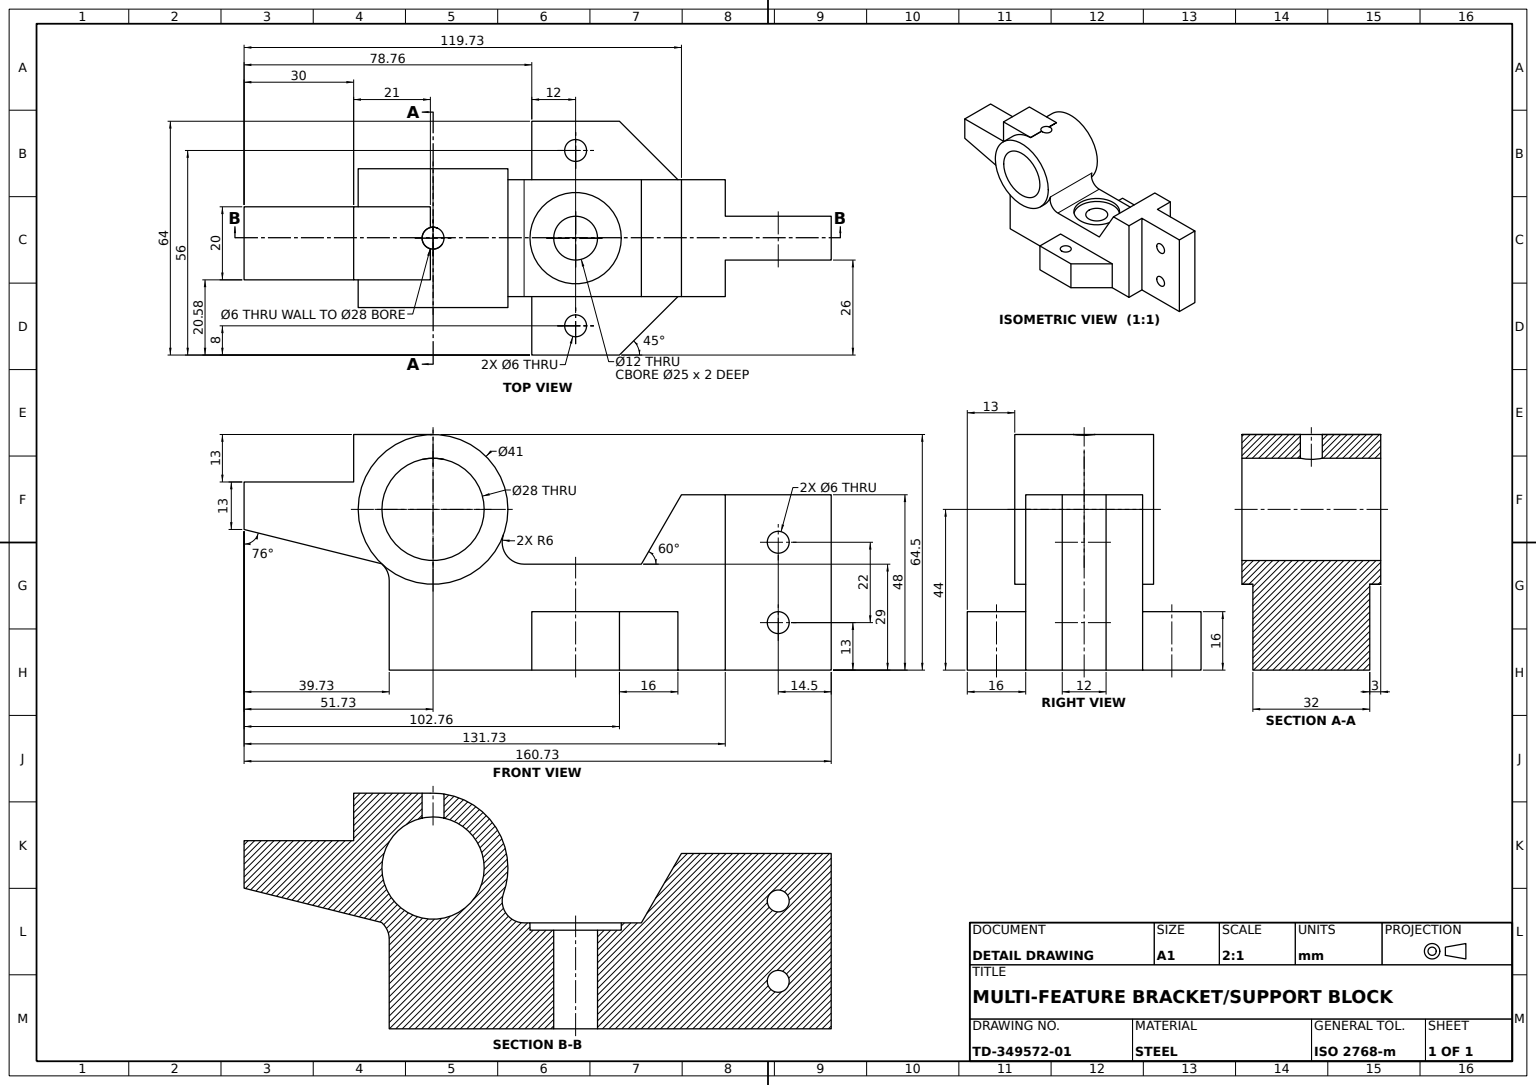
SolidWorks part; units mm, degrees
material "Plain Carbon Steel"
ref_plane "Front Plane" through (0, 0, 0) normal (0, 0, 1) x (1, 0, 0)
ref_plane "Top Plane" through (0, 0, 0) normal (0, 1, 0) x (1, 0, 0)
ref_plane "Right Plane" through (0, 0, 0) normal (1, 0, 0) x (0, 0, -1)
sketch "Pedestal Profile Sketch" plane through (0, 0, 0) normal (0, 0, 1) x (1, 0, 0)
  line L0 (-46, 0) -> (46, 0)
  line L1 (-46, 0) -> (-46, 24.5513)
  line L2 (46, 0) -> (46, 48)
  line L3 (46, 48) -> (34, 48)
  line L4 (-9.0751, 29) -> (23.0303, 29)
  line L5 (34, 48) -> (23.0303, 29)
  line L7 (-46, 29) -> (46, 29) construction
  arc A0 (-14.7185, 37.0377) -> (-47.9245, 28.9548) centre (-34, 44) ccw
  circle A1 centre (-34, 44) radius 14
  arc A2 (-46, 24.5513) -> (-47.9245, 28.9548) centre (-52, 24.5513) ccw
  arc A3 (-9.0751, 29) -> (-14.7185, 37.0377) centre (-9.0751, 35) cw
  point P7 (0, 0)
  dimension "D1" = 41
  dimension "D2" = 28
  dimension "D10" = 6
  dimension "D3" = 46
  dimension "D4" = 12
  dimension "D5" = 44
  dimension "D6" = 48
  dimension "D7" = 12
  dimension "D9" = 30
  dimension "D8" = 29
extrude "Pedestal Body" add sketch "Pedestal Profile Sketch" along normal blind 32
sketch "Vertical Bore Sketch" plane through (0, 29, 0) normal (0, 1, 0) x (1, 0, 0)
  line L0 (23.0303, -32) -> (23.0303, 0) construction
  line L1 (23.0303, 0) -> (-9.0751, 0) construction
  circle A1 centre (5.0303, -16) radius 6
  dimension "D1" = 12
  dimension "D2" = 18
  dimension "D3" = 16
extrude "Vertical Bore Ø16" cut sketch "Vertical Bore Sketch" against normal blind 32
sketch "Counterbore Sketch" plane through (0, 29, 0) normal (0, 1, 0) x (1, 0, 0)
  circle A0 centre (5.0303, -16) radius 12.5
  dimension "D1" = 25
extrude "Counterbore Ø25x2" cut sketch "Counterbore Sketch" against normal blind 2
sketch "Side Mounting Block Sketch" plane through (0, 48, 0) normal (0, 1, 0) x (1, 0, 0)
  line L0 (46, -32) -> (46, 0) construction
  line L1 (46, -10) -> (75, -10)
  line L2 (46, -10) -> (46, -22)
  line L3 (46, -22) -> (75, -22)
  line L4 (75, -10) -> (75, -22)
  line L5 (46, 0) -> (34, 0) construction
  line L6 (46, -32) -> (34, -32) construction
  dimension "D1" = 29
  dimension "D2" = 10
  dimension "D3" = 10
extrude "Side Mounting Block" add sketch "Side Mounting Block Sketch" against normal blind 48
sketch "Block Mounting Holes Sketch" plane through (0, 0, 22) normal (0, 0, 1) x (1, 0, 0)
  line L0 (46, 48) -> (75, 48) construction
  line L1 (46, 0) -> (75, 0) construction
  line L2 (75, 0) -> (75, 48) construction
  circle A0 centre (60.5, 35) radius 3
  circle A1 centre (60.5, 13) radius 3
  dimension "D1" = 6
  dimension "D2" = 6
  dimension "D3" = 22
  dimension "D4" = 13
  dimension "D5" = 13
  dimension "D6" = 14.5
extrude "Block Mounting Holes 2xØ6" cut sketch "Block Mounting Holes Sketch" against normal blind 48
sketch "T-Slot Flange Sketch" plane through (0, 0, 0) normal (0, -1, 0) x (1, 0, 0)
  line L0 (34, 32) -> (34, 0) construction
  line L1 (75, 22) -> (75, 10) construction
  line L2 (23.0303, 0) -> (-9.0751, 0) construction
  line L3 (23.0303, 32) -> (-9.0751, 32) construction
  line L4 (-6.9697, -16) -> (-6.9697, 0)
  line L5 (17.0303, -16) -> (-6.9697, -16)
  line L6 (-6.9697, 0) -> (33.0303, 0)
  line L7 (34, 0) -> (23.0303, 0) construction
  line L8 (17.0303, 48) -> (-6.9697, 48)
  line L9 (33.0303, 0) -> (17.0303, -16)
  line L10 (17.0303, 48) -> (33.0303, 32)
  line L11 (34, 32) -> (23.0303, 32) construction
  line L12 (33.0303, 32) -> (-6.9697, 32)
  line L13 (-6.9697, 32) -> (-6.9697, 48)
  circle A0 centre (5.0303, -8) radius 3
  circle A1 centre (5.0303, 40) radius 3
  point P8 (75, 16)
  point P9 (5.0303, 48)
  point P10 (5.0303, -16)
  dimension "D1" = 6
  dimension "D2" = 6
  dimension "D3" = 48
  dimension "D4" = 28.9697
  dimension "D5" = 24
  dimension "D6" = 24
  dimension "D9" = 12
  dimension "D7" = 12
  dimension "D8" = 0
  dimension "D10" = 16
  dimension "D11" = 16
  dimension "D12" = 16
  dimension "D13" = 16
extrude "T-Slot Flange" add sketch "T-Slot Flange Sketch" against normal blind 16
ref_plane "Plane1" through (0, 64.5, 0) normal (0, 1, 0) x (1, 0, 0)
sketch "Top Hole Sketch" plane through (0, 64.5, 0) normal (0, 1, 0) x (1, 0, 0)
  line L0 (-13.5, 0) -> (-54.5, 0) construction
  line L1 (-54.5, 0) -> (-54.5, -32) construction
  circle A0 centre (-34, -16) radius 3
  dimension "D1" = 6
  dimension "D2" = 16
  dimension "D3" = 20.5
extrude "Top Hole Ø6" cut sketch "Top Hole Sketch" against normal blind 16
sketch "Upper Arm Block Sketch" plane through (0, 64.5, 0) normal (0, 1, 0) x (1, 0, 0)
  line L0 (-13.5, 0) -> (-54.5, 0) construction
  line L1 (-34.7329, -7.4161) -> (-55.7329, -7.4161)
  line L2 (-34.7329, -7.4161) -> (-34.7329, -13.0909)
  line L3 (-34.7329, -27.4161) -> (-55.7329, -27.4161)
  line L4 (-55.7329, -7.4161) -> (-55.7329, -27.4161)
  line L5 (-54.5, 0) -> (-54.5, -32) construction
  line L6 (-34.7329, -18.9091) -> (-34.7329, -27.4161)
  arc A0 (-34.7329, -13.0909) -> (-34.7329, -18.9091) centre (-34, -16) ccw
  dimension "D5" = 6
  dimension "D1" = 21
  dimension "D2" = 20
  dimension "D3" = 7.4161
  dimension "D4" = 1.2329
extrude "Upper Arm Block" add sketch "Upper Arm Block Sketch" against normal blind 13
sketch "Trunnion Bore Sketch A" plane through (0, 0, 32) normal (0, 0, 1) x (1, 0, 0)
  circle A0 centre (-34, 44) radius 14
  dimension "D1" = 28
extrude "Trunnion Bore Ø28 A" cut sketch "Trunnion Bore Sketch A" against normal blind 60
sketch "Upper Arm Extension Sketch" plane through (0, 51.5, 0) normal (0, -1, 0) x (1, 0, 0)
  line L0 (-46.7329, 7.4161) -> (-46.7329, 27.4161)
  line L1 (-53.0788, 7.4161) -> (-34.7329, 7.4161) construction
  line L2 (-55.7329, 27.4161) -> (-34.7329, 27.4161) construction
  line L3 (-55.7329, 7.4161) -> (-55.7329, 27.4161) construction
  line L5 (-46.7329, 7.4161) -> (-85.7329, 7.4161)
  line L6 (-46.7329, 7.4161) -> (-46.7329, 27.4161)
  line L7 (-46.7329, 27.4161) -> (-85.7329, 27.4161)
  line L8 (-85.7329, 7.4161) -> (-85.7329, 27.4161)
  line M4 (-55.7329, 7.4161) -> (-53.0788, 7.4161)
  line M5 (-53.0788, 7.4161) -> (-53.0788, 27.4161)
  line M6 (-53.0788, 27.4161) -> (-55.7329, 27.4161)
  line M7 (-55.7329, 27.4161) -> (-55.7329, 7.4161)
  dimension "D1" = 9
  dimension "D2" = 39
  dimension "D3" = 20
extrude "Upper Arm Extension" add sketch "Upper Arm Extension Sketch" along normal blind 13 contours L8 L5 L7 M7 | L0 L7 L5 M5 | M7 M4 M5 M6
sketch "Angled Side Lug Sketch" plane through (0, 0, 27.4161) normal (0, 0, 1) x (1, 0, 0)
  line L0 (-85.7329, 38.5) -> (-48.097, 29.1163)
  line L1 (-85.7329, 38.5) -> (-53.7484, 38.5)
  arc A0 (-48.097, 29.1163) -> (-53.7484, 38.5) centre (-34, 44) cw
  dimension "D3" = 20.5
  dimension "D1" = 14
  dimension "D2" = 29.1163
  dimension "D4" = 53.7484
extrude "Angled Side Lug" add sketch "Angled Side Lug Sketch" against normal blind 20
sketch "Trunnion Bore Sketch B" plane through (0, 0, 32) normal (0, 0, 1) x (1, 0, 0)
  circle A0 centre (-34, 44) radius 14
  dimension "D1" = 28
extrude "Trunnion Bore Ø28 B" cut sketch "Trunnion Bore Sketch B" against normal blind 60
sketch "Bore Collar Sketch A" plane through (0, 0, 32) normal (0, 0, 1) x (1, 0, 0)
  circle A0 centre (-34, 44) radius 14
  circle A1 centre (-34, 44) radius 20.5
  dimension "D1" = 41
  dimension "D2" = 28
extrude "Bore Collar Ø41x3 A" add sketch "Bore Collar Sketch A" along normal blind 3
sketch "Bore Collar Sketch B" plane through (0, 0, 0) normal (0, 0, -1) x (-1, 0, 0)
  circle A0 centre (34, 44) radius 14
  circle A1 centre (34, 44) radius 20.5
  dimension "D1" = 28
  dimension "D2" = 41
extrude "Bore Collar Ø41x3 B" add sketch "Bore Collar Sketch B" along normal blind 3
